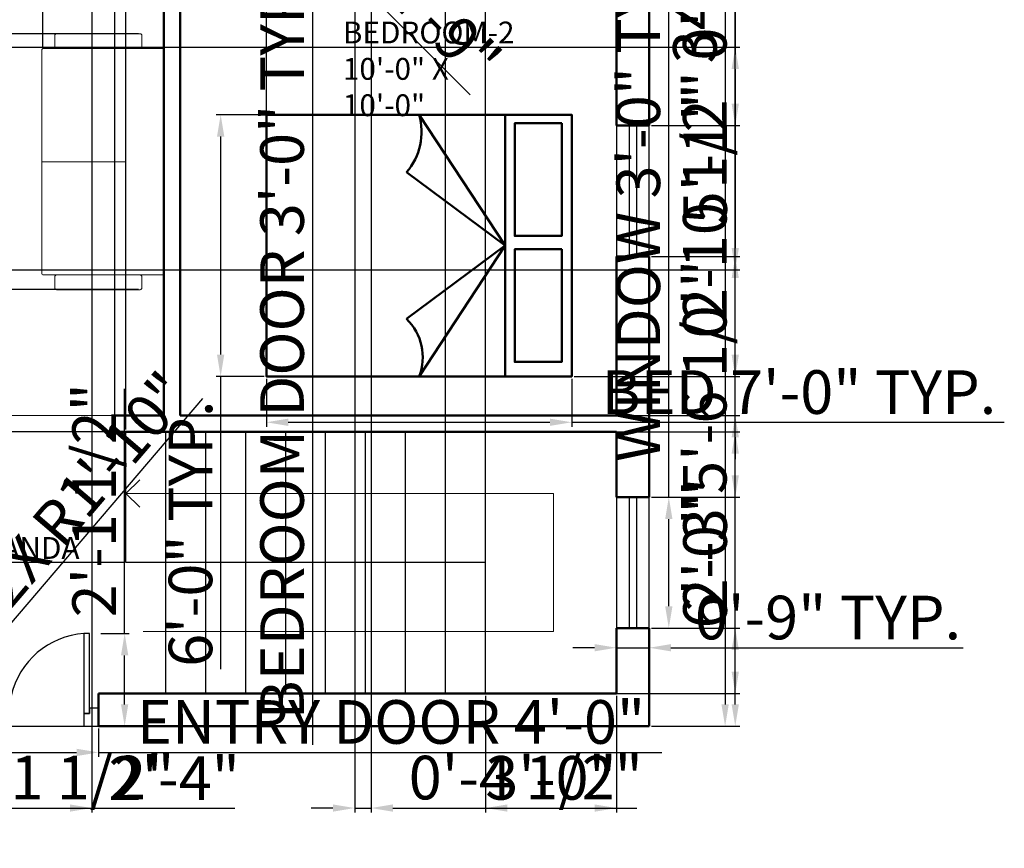
# Model space of a CAD drawing. Units: inches. Extents: x 1086 to 1501, y 383 to 973.
# Tile 2 of 7: x 1230 to 1501, y 383 to 611. Entities that reach past the tile are written whole.
import ezdxf

# ---------------------------------------------------------------- set-up
doc = ezdxf.new("R2010")
doc.units = ezdxf.units.IN
for name, color, linetype, lineweight in [('A-ANNO-DIMS', 2, 'Continuous', 18), ('A-ANNO-SYMB', 201, 'Continuous', 18), ('A-AREA-IDEN', 7, 'Continuous', 25), ('door', 10, 'Continuous', 25), ('furniture', 255, 'Continuous', 18), ('opening', 219, 'Continuous', 18), ('staircase', 201, 'Continuous', 25), ('wall', 7, 'Continuous', 50), ('window', 81, 'Continuous', 25)]:
    doc.layers.add(name, color=color, linetype=linetype, lineweight=lineweight)
doc.styles.get("Standard").update_dxf_attribs({"font": 'arial.ttf'})
doc.dimstyles.new('ISO-25', dxfattribs={"dimtxt": 12, "dimasz": 6, "dimexe": 1.25, "dimexo": 0.625, "dimtad": 1, "dimdec": 1, "dimlunit": 3, "dimtxsty": 'Standard', "dimcen": 2.5, "dimadec": 0, "dimazin": 0, "dimtfac": 1, "dimtdec": 1, "dimtmove": 0, "dimatfit": 3, "dimfxl": 1, "dimarcsym": 0})

# ---------------------------------------------------------------- blocks, each defined once
blk = doc.blocks.new('d3')
at = {"layer": 'door'}
blk.add_line((1743.18, 564.73), (1791.18, 564.73), dxfattribs=at)
for points in [[(1745.68, 568.23), (1747.18, 568.23), (1747.18, 590.23), (1745.68, 590.23)], [(1787.18, 568.23), (1788.68, 568.23), (1788.68, 590.23), (1787.18, 590.23)]]:
    blk.add_lwpolyline(points, close=True, dxfattribs=at)
for points in [[(1747.18, 564.73), (1743.18, 564.73), (1743.18, 569.73), (1745.68, 569.73), (1745.68, 568.23), (1747.18, 568.23), (1747.18, 564.73)], [(1787.18, 564.73), (1791.18, 564.73), (1791.18, 569.73), (1788.68, 569.73), (1788.68, 568.23), (1787.18, 568.23), (1787.18, 564.73)]]:
    blk.add_lwpolyline(points, dxfattribs=at)
for centre, start, end in [((1745.68, 568.23), 12.8362, 86.0995), ((1788.68, 568.23), 93.9005, 167.1638)]:
    blk.add_arc(centre, 22.05, start, end, dxfattribs=at)
blk = doc.blocks.new('w1')
at = {"layer": 'window'}
for p, q in [((1475.33, 845.32), (1475.33, 809.32)), ((1477.33, 845.32), (1477.33, 809.32))]:
    blk.add_line(p, q, dxfattribs=at)
blk.add_lwpolyline([(1471.83, 809.32), (1480.83, 809.32), (1480.83, 845.32), (1471.83, 845.32)], close=True, dxfattribs=at)
blk = doc.blocks.new('bed')
at = {"layer": 'wall'}
for p, q in [((1549.71, 859.44), (1621.71, 859.44)), ((1585.71, 859.44), (1549.71, 835.76)), ((1585.71, 859.44), (1565.54, 832.3)), ((1585.71, 859.44), (1621.71, 835.76)), ((1585.71, 859.44), (1605.88, 832.3))]:
    blk.add_line(p, q, dxfattribs=at)
for points in [[(1549.71, 793.76), (1621.71, 793.76), (1621.71, 877.76), (1549.71, 877.76)], [(1552.04, 875), (1583.04, 875), (1583.04, 862.08), (1552.04, 862.08)], [(1586.71, 875), (1617.71, 875), (1617.71, 862.08), (1586.71, 862.08)]]:
    blk.add_lwpolyline(points, close=True, dxfattribs=at)
for centre, radius, start, end in [((1554.45, 819.53), 16.91, 49.0428, 106.2967), ((1616.39, 822.13), 14.63, 68.7093, 135.9513)]:
    blk.add_arc(centre, radius, start, end, dxfattribs=at)
blk = doc.blocks.new('*D10')
at = {"layer": 'A-ANNO-DIMS', "color": 0, "lineweight": -2, "transparency": 16777216}
for p, q in [((1404.05, 835.21), (1425.57, 835.21)), ((1424.32, 829.21), (1424.32, 422.21)), ((1404.05, 416.21), (1425.57, 416.21))]:
    blk.add_line(p, q, dxfattribs=at)
at = {"layer": 'A-ANNO-DIMS', "color": 0, "transparency": 16777216}
for points in [[(1423.32, 829.21), (1425.32, 829.21), (1424.32, 835.21)], [(1423.32, 422.21), (1425.32, 422.21), (1424.32, 416.21)]]:
    blk.add_solid(points, dxfattribs=at)
at = {"layer": 'Defpoints', "color": 0, "transparency": 16777216}
for p in [(1403.43, 835.21), (1403.43, 416.21), (1424.32, 416.21)]:
    blk.add_point(p, dxfattribs=at)
at = {"layer": 'A-ANNO-DIMS', "color": 0, "transparency": 16777216, "insert": (1417.56, 625.71), "char_height": 12, "attachment_point": 5, "rotation": 90}
blk.add_mtext('34\'-11"', dxfattribs=at)
blk = doc.blocks.new('*D13')
at = {"layer": 'A-ANNO-DIMS', "color": 0, "lineweight": -2, "transparency": 16777216}
for p, q in [((1408.83, 479.21), (1408.83, 638.31)), ((1404.05, 479.21), (1410.08, 479.21)), ((1408.83, 449.21), (1408.83, 473.21)), ((1404.05, 443.21), (1410.08, 443.21))]:
    blk.add_line(p, q, dxfattribs=at)
at = {"layer": 'A-ANNO-DIMS', "color": 0, "transparency": 16777216}
for points in [[(1407.83, 473.21), (1409.83, 473.21), (1408.83, 479.21)], [(1407.83, 449.21), (1409.83, 449.21), (1408.83, 443.21)]]:
    blk.add_solid(points, dxfattribs=at)
at = {"layer": 'Defpoints', "color": 0, "transparency": 16777216}
for p in [(1403.43, 479.21), (1408.83, 479.21), (1403.43, 443.21)]:
    blk.add_point(p, dxfattribs=at)
at = {"layer": 'A-ANNO-DIMS', "color": 0, "transparency": 16777216, "insert": (1401.99, 561.76), "char_height": 12, "attachment_point": 5, "rotation": 90}
blk.add_mtext('WINDOW 3\'-0" TYP.', dxfattribs=at)
blk = doc.blocks.new('*D14')
at = {"layer": 'A-ANNO-DIMS', "color": 0, "lineweight": -2, "transparency": 16777216}
for p, q in [((1394.43, 442.58), (1394.43, 436.56)), ((1403.43, 442.58), (1403.43, 436.56)), ((1388.43, 437.81), (1382.43, 437.81)), ((1394.43, 437.81), (1403.43, 437.81)), ((1409.43, 437.81), (1489.83, 437.81))]:
    blk.add_line(p, q, dxfattribs=at)
at = {"layer": 'A-ANNO-DIMS', "color": 0, "transparency": 16777216}
for points in [[(1388.43, 438.81), (1388.43, 436.81), (1394.43, 437.81)], [(1409.43, 438.81), (1409.43, 436.81), (1403.43, 437.81)]]:
    blk.add_solid(points, dxfattribs=at)
at = {"layer": 'Defpoints', "color": 0, "transparency": 16777216}
for p in [(1394.43, 443.21), (1403.43, 443.21), (1403.43, 437.81)]:
    blk.add_point(p, dxfattribs=at)
at = {"layer": 'A-ANNO-DIMS', "color": 0, "transparency": 16777216, "insert": (1452.63, 444.56), "char_height": 12, "attachment_point": 5}
blk.add_mtext('0\'-9" TYP.', dxfattribs=at)
blk = doc.blocks.new('*D19')
at = {"layer": 'A-ANNO-DIMS', "color": 0, "lineweight": -2, "transparency": 16777216}
for p, q in [((1306.05, 673.21), (1312.08, 673.21)), ((1310.83, 667.21), (1310.83, 643.21)), ((1306.05, 637.21), (1312.08, 637.21)), ((1310.83, 637.21), (1310.83, 411.12))]:
    blk.add_line(p, q, dxfattribs=at)
at = {"layer": 'A-ANNO-DIMS', "color": 0, "transparency": 16777216}
for points in [[(1309.83, 667.21), (1311.83, 667.21), (1310.83, 673.21)], [(1309.83, 643.21), (1311.83, 643.21), (1310.83, 637.21)]]:
    blk.add_solid(points, dxfattribs=at)
at = {"layer": 'Defpoints', "color": 0, "transparency": 16777216}
for p in [(1305.43, 673.21), (1305.43, 637.21), (1310.83, 637.21)]:
    blk.add_point(p, dxfattribs=at)
at = {"layer": 'A-ANNO-DIMS', "color": 0, "transparency": 16777216, "insert": (1303.99, 521.16), "char_height": 12, "attachment_point": 5, "rotation": 90}
blk.add_mtext('BEDROOM DOOR 3\'-0" TYP.', dxfattribs=at)
blk = doc.blocks.new('*D21')
at = {"layer": 'A-ANNO-DIMS', "color": 0, "lineweight": -2, "transparency": 16777216}
for p, q in [((1203.93, 415.58), (1203.93, 407.76)), ((1251.93, 415.58), (1251.93, 407.76)), ((1209.93, 409.01), (1245.93, 409.01)), ((1251.93, 409.01), (1406.87, 409.01))]:
    blk.add_line(p, q, dxfattribs=at)
at = {"layer": 'A-ANNO-DIMS', "color": 0, "transparency": 16777216}
for points in [[(1209.93, 410.01), (1209.93, 408.01), (1203.93, 409.01)], [(1245.93, 410.01), (1245.93, 408.01), (1251.93, 409.01)]]:
    blk.add_solid(points, dxfattribs=at)
at = {"layer": 'Defpoints', "color": 0, "transparency": 16777216}
for p in [(1203.93, 416.21), (1251.93, 416.21), (1251.93, 409.01)]:
    blk.add_point(p, dxfattribs=at)
at = {"layer": 'A-ANNO-DIMS', "color": 0, "transparency": 16777216, "insert": (1332.4, 415.84), "char_height": 12, "attachment_point": 5}
blk.add_mtext('ENTRY DOOR 4\'-0"', dxfattribs=at)
blk = doc.blocks.new('*D22')
at = {"layer": 'A-ANNO-DIMS', "color": 0, "lineweight": -2, "transparency": 16777216}
for p, q in [((1259.13, 441.71), (1259.13, 509.02)), ((1252.55, 441.71), (1260.38, 441.71)), ((1259.13, 422.21), (1259.13, 435.71)), ((1252.55, 416.21), (1260.38, 416.21))]:
    blk.add_line(p, q, dxfattribs=at)
at = {"layer": 'A-ANNO-DIMS', "color": 0, "transparency": 16777216}
for points in [[(1258.13, 435.71), (1260.13, 435.71), (1259.13, 441.71)], [(1258.13, 422.21), (1260.13, 422.21), (1259.13, 416.21)]]:
    blk.add_solid(points, dxfattribs=at)
at = {"layer": 'Defpoints', "color": 0, "transparency": 16777216}
for p in [(1251.93, 441.71), (1259.13, 441.71), (1251.93, 416.21)]:
    blk.add_point(p, dxfattribs=at)
at = {"layer": 'A-ANNO-DIMS', "color": 0, "transparency": 16777216, "insert": (1252.3, 478.36), "char_height": 12, "attachment_point": 5, "rotation": 90}
blk.add_mtext('2\'-1 1/2"', dxfattribs=at)
blk = doc.blocks.new('*D23')
at = {"layer": 'A-ANNO-DIMS', "color": 0, "lineweight": -2, "transparency": 16777216}
for p, q in [((1298.14, 511.79), (1298.14, 498.57)), ((1382.14, 511.79), (1382.14, 498.57)), ((1304.14, 499.82), (1376.14, 499.82)), ((1382.14, 499.82), (1501.13, 499.82))]:
    blk.add_line(p, q, dxfattribs=at)
at = {"layer": 'A-ANNO-DIMS', "color": 0, "transparency": 16777216}
for points in [[(1304.14, 500.82), (1304.14, 498.82), (1298.14, 499.82)], [(1376.14, 500.82), (1376.14, 498.82), (1382.14, 499.82)]]:
    blk.add_solid(points, dxfattribs=at)
at = {"layer": 'Defpoints', "color": 0, "transparency": 16777216}
for p in [(1298.14, 512.42), (1382.14, 512.42), (1382.14, 499.82)]:
    blk.add_point(p, dxfattribs=at)
at = {"layer": 'A-ANNO-DIMS', "color": 0, "transparency": 16777216, "insert": (1444.63, 506.57), "char_height": 12, "attachment_point": 5}
blk.add_mtext('BED 7\'-0" TYP.', dxfattribs=at)
blk = doc.blocks.new('*D24')
at = {"layer": 'A-ANNO-DIMS', "color": 0, "lineweight": -2, "transparency": 16777216}
for p, q in [((1297.51, 584.42), (1284.29, 584.42)), ((1285.54, 578.42), (1285.54, 518.42)), ((1297.51, 512.42), (1284.29, 512.42)), ((1285.54, 512.42), (1285.54, 431.95))]:
    blk.add_line(p, q, dxfattribs=at)
at = {"layer": 'A-ANNO-DIMS', "color": 0, "transparency": 16777216}
for points in [[(1284.54, 578.42), (1286.54, 578.42), (1285.54, 584.42)], [(1284.54, 518.42), (1286.54, 518.42), (1285.54, 512.42)]]:
    blk.add_solid(points, dxfattribs=at)
at = {"layer": 'Defpoints', "color": 0, "transparency": 16777216}
for p in [(1298.14, 584.42), (1285.54, 512.42), (1298.14, 512.42)]:
    blk.add_point(p, dxfattribs=at)
at = {"layer": 'A-ANNO-DIMS', "color": 0, "transparency": 16777216, "insert": (1278.79, 469.18), "char_height": 12, "attachment_point": 5, "rotation": 90}
blk.add_mtext('6\'-0" TYP.', dxfattribs=at)
blk = doc.blocks.new('*D34')
at = {"layer": 'A-ANNO-DIMS', "color": 0, "lineweight": -2, "transparency": 16777216}
for p, q in [((1427.11, 443.21), (1427.11, 482.56)), ((1404.05, 443.21), (1428.36, 443.21)), ((1427.11, 422.21), (1427.11, 437.21)), ((1404.05, 416.21), (1428.36, 416.21))]:
    blk.add_line(p, q, dxfattribs=at)
at = {"layer": 'A-ANNO-DIMS', "color": 0, "transparency": 16777216}
for points in [[(1426.11, 437.21), (1428.11, 437.21), (1427.11, 443.21)], [(1426.11, 422.21), (1428.11, 422.21), (1427.11, 416.21)]]:
    blk.add_solid(points, dxfattribs=at)
at = {"layer": 'Defpoints', "color": 0, "transparency": 16777216}
for p in [(1403.43, 443.21), (1427.11, 443.21), (1403.43, 416.21)]:
    blk.add_point(p, dxfattribs=at)
at = {"layer": 'A-ANNO-DIMS', "color": 0, "transparency": 16777216, "insert": (1420.36, 465.88), "char_height": 12, "attachment_point": 5, "rotation": 90}
blk.add_mtext('2\'-3"', dxfattribs=at)
blk = doc.blocks.new('*D35')
at = {"layer": 'A-ANNO-DIMS', "color": 0, "lineweight": -2, "transparency": 16777216}
for p, q in [((1404.05, 545.46), (1428.36, 545.46)), ((1427.11, 485.21), (1427.11, 539.46)), ((1404.05, 479.21), (1428.36, 479.21))]:
    blk.add_line(p, q, dxfattribs=at)
at = {"layer": 'A-ANNO-DIMS', "color": 0, "transparency": 16777216}
for points in [[(1426.11, 539.46), (1428.11, 539.46), (1427.11, 545.46)], [(1426.11, 485.21), (1428.11, 485.21), (1427.11, 479.21)]]:
    blk.add_solid(points, dxfattribs=at)
at = {"layer": 'Defpoints', "color": 0, "transparency": 16777216}
for p in [(1403.43, 545.46), (1427.11, 545.46), (1403.43, 479.21)]:
    blk.add_point(p, dxfattribs=at)
at = {"layer": 'A-ANNO-DIMS', "color": 0, "transparency": 16777216, "insert": (1420.28, 512.33), "char_height": 12, "attachment_point": 5, "rotation": 90}
blk.add_mtext('5\'-6 1/2"', dxfattribs=at)
blk = doc.blocks.new('*D36')
at = {"layer": 'A-ANNO-DIMS', "color": 0, "lineweight": -2, "transparency": 16777216}
for p, q in [((1427.11, 641.71), (1427.11, 708.82)), ((1404.05, 641.71), (1428.36, 641.71)), ((1427.11, 587.46), (1427.11, 635.71)), ((1404.05, 581.46), (1428.36, 581.46))]:
    blk.add_line(p, q, dxfattribs=at)
at = {"layer": 'A-ANNO-DIMS', "color": 0, "transparency": 16777216}
for points in [[(1426.11, 635.71), (1428.11, 635.71), (1427.11, 641.71)], [(1426.11, 587.46), (1428.11, 587.46), (1427.11, 581.46)]]:
    blk.add_solid(points, dxfattribs=at)
at = {"layer": 'Defpoints', "color": 0, "transparency": 16777216}
for p in [(1403.43, 641.71), (1427.11, 641.71), (1403.43, 581.46)]:
    blk.add_point(p, dxfattribs=at)
at = {"layer": 'A-ANNO-DIMS', "color": 0, "transparency": 16777216, "insert": (1420.28, 678.26), "char_height": 12, "attachment_point": 5, "rotation": 90}
blk.add_mtext('5\'-0 1/2"', dxfattribs=at)
blk = doc.blocks.new('*D39')
at = {"layer": 'A-ANNO-DIMS', "color": 0, "lineweight": -2, "transparency": 16777216}
for p, q in [((1178.43, 415.58), (1178.43, 392.46)), ((1203.93, 415.58), (1203.93, 392.46)), ((1184.43, 393.71), (1197.93, 393.71)), ((1203.93, 393.71), (1271.25, 393.71))]:
    blk.add_line(p, q, dxfattribs=at)
at = {"layer": 'A-ANNO-DIMS', "color": 0, "transparency": 16777216}
for points in [[(1184.43, 394.71), (1184.43, 392.71), (1178.43, 393.71)], [(1197.93, 394.71), (1197.93, 392.71), (1203.93, 393.71)]]:
    blk.add_solid(points, dxfattribs=at)
at = {"layer": 'Defpoints', "color": 0, "transparency": 16777216}
for p in [(1178.43, 416.21), (1203.93, 416.21), (1203.93, 393.71)]:
    blk.add_point(p, dxfattribs=at)
at = {"layer": 'A-ANNO-DIMS', "color": 0, "transparency": 16777216, "insert": (1240.59, 400.54), "char_height": 12, "attachment_point": 5}
blk.add_mtext('2\'-1 1/2"', dxfattribs=at)
blk = doc.blocks.new('*D40')
at = {"layer": 'A-ANNO-DIMS', "color": 0, "lineweight": -2, "transparency": 16777216}
for p, q in [((1142.43, 502.33), (1142.43, 867.19)), ((1269.93, 502.33), (1269.93, 867.19)), ((1148.43, 865.94), (1263.93, 865.94))]:
    blk.add_line(p, q, dxfattribs=at)
at = {"layer": 'A-ANNO-DIMS', "color": 0, "transparency": 16777216}
for points in [[(1148.43, 866.94), (1148.43, 864.94), (1142.43, 865.94)], [(1263.93, 866.94), (1263.93, 864.94), (1269.93, 865.94)]]:
    blk.add_solid(points, dxfattribs=at)
at = {"layer": 'Defpoints', "color": 0, "transparency": 16777216}
for p in [(1269.93, 865.94), (1142.43, 501.71), (1269.93, 501.71)]:
    blk.add_point(p, dxfattribs=at)
at = {"layer": 'A-ANNO-DIMS', "color": 0, "transparency": 16777216, "insert": (1206.18, 872.77), "char_height": 12, "attachment_point": 5}
blk.add_mtext('10\'-7 1/2"', dxfattribs=at)
blk = doc.blocks.new('*D42')
at = {"layer": 'A-ANNO-DIMS', "color": 0, "lineweight": -2, "transparency": 16777216}
for p, q in [((1256.43, 502.33), (1256.43, 867.19)), ((1269.93, 502.33), (1269.93, 867.19)), ((1262.43, 865.94), (1263.93, 865.94)), ((1269.93, 865.94), (1335.91, 865.94))]:
    blk.add_line(p, q, dxfattribs=at)
at = {"layer": 'A-ANNO-DIMS', "color": 0, "transparency": 16777216}
for points in [[(1262.43, 866.94), (1262.43, 864.94), (1256.43, 865.94)], [(1263.93, 866.94), (1263.93, 864.94), (1269.93, 865.94)]]:
    blk.add_solid(points, dxfattribs=at)
at = {"layer": 'Defpoints', "color": 0, "transparency": 16777216}
for p in [(1269.93, 865.94), (1256.43, 501.71), (1269.93, 501.71)]:
    blk.add_point(p, dxfattribs=at)
at = {"layer": 'A-ANNO-DIMS', "color": 0, "transparency": 16777216, "insert": (1305.92, 872.77), "char_height": 12, "attachment_point": 5}
blk.add_mtext('1\'-1 1/2"', dxfattribs=at)
blk = doc.blocks.new('*D43')
at = {"layer": 'A-ANNO-DIMS', "color": 0, "lineweight": -2, "transparency": 16777216}
for p, q in [((1208.43, 497.83), (1208.43, 867.19)), ((1256.43, 497.83), (1256.43, 867.19)), ((1214.43, 865.94), (1250.43, 865.94))]:
    blk.add_line(p, q, dxfattribs=at)
at = {"layer": 'A-ANNO-DIMS', "color": 0, "transparency": 16777216}
for points in [[(1214.43, 866.94), (1214.43, 864.94), (1208.43, 865.94)], [(1250.43, 866.94), (1250.43, 864.94), (1256.43, 865.94)]]:
    blk.add_solid(points, dxfattribs=at)
at = {"layer": 'Defpoints', "color": 0, "transparency": 16777216}
for p in [(1256.43, 865.94), (1208.43, 497.21), (1256.43, 497.21)]:
    blk.add_point(p, dxfattribs=at)
at = {"layer": 'A-ANNO-DIMS', "color": 0, "transparency": 16777216, "insert": (1232.43, 872.69), "char_height": 12, "attachment_point": 5}
blk.add_mtext('4\'-0"', dxfattribs=at)
blk = doc.blocks.new('*D44')
at = {"layer": 'A-ANNO-DIMS', "color": 0, "lineweight": -2, "transparency": 16777216}
for p, q in [((1258.8, 497.21), (1109.68, 497.21)), ((1110.93, 491.21), (1110.93, 467.21)), ((1258.8, 461.21), (1109.68, 461.21))]:
    blk.add_line(p, q, dxfattribs=at)
at = {"layer": 'A-ANNO-DIMS', "color": 0, "transparency": 16777216}
for points in [[(1109.93, 491.21), (1111.93, 491.21), (1110.93, 497.21)], [(1109.93, 467.21), (1111.93, 467.21), (1110.93, 461.21)]]:
    blk.add_solid(points, dxfattribs=at)
at = {"layer": 'Defpoints', "color": 0, "transparency": 16777216}
for p in [(1259.43, 497.21), (1110.93, 461.21), (1259.43, 461.21)]:
    blk.add_point(p, dxfattribs=at)
at = {"layer": 'A-ANNO-DIMS', "color": 0, "transparency": 16777216, "insert": (1104.17, 479.21), "char_height": 12, "attachment_point": 5, "rotation": 90}
blk.add_mtext('3\'-0"', dxfattribs=at)
blk = doc.blocks.new('*D45')
at = {"layer": 'A-ANNO-DIMS', "color": 0, "lineweight": -2, "transparency": 16777216}
for p, q in [((1259.43, 497.83), (1259.43, 867.19)), ((1358.43, 497.83), (1358.43, 867.19)), ((1265.43, 865.94), (1352.43, 865.94))]:
    blk.add_line(p, q, dxfattribs=at)
at = {"layer": 'A-ANNO-DIMS', "color": 0, "transparency": 16777216}
for points in [[(1265.43, 866.94), (1265.43, 864.94), (1259.43, 865.94)], [(1352.43, 866.94), (1352.43, 864.94), (1358.43, 865.94)]]:
    blk.add_solid(points, dxfattribs=at)
at = {"layer": 'Defpoints', "color": 0, "transparency": 16777216}
for p in [(1358.43, 865.94), (1259.43, 497.21), (1358.43, 497.21)]:
    blk.add_point(p, dxfattribs=at)
at = {"layer": 'A-ANNO-DIMS', "color": 0, "transparency": 16777216, "insert": (1308.93, 872.7), "char_height": 12, "attachment_point": 5}
blk.add_mtext('8\'-3"', dxfattribs=at)
blk = doc.blocks.new('*D46')
at = {"layer": 'A-ANNO-DIMS', "color": 0, "lineweight": -2, "transparency": 16777216}
for p, q in [((1358.43, 424.58), (1358.43, 392.46)), ((1394.43, 424.58), (1394.43, 392.46)), ((1364.43, 393.71), (1388.43, 393.71))]:
    blk.add_line(p, q, dxfattribs=at)
at = {"layer": 'A-ANNO-DIMS', "color": 0, "transparency": 16777216}
for points in [[(1364.43, 394.71), (1364.43, 392.71), (1358.43, 393.71)], [(1388.43, 394.71), (1388.43, 392.71), (1394.43, 393.71)]]:
    blk.add_solid(points, dxfattribs=at)
at = {"layer": 'Defpoints', "color": 0, "transparency": 16777216}
for p in [(1358.43, 425.21), (1394.43, 425.21), (1394.43, 393.71)]:
    blk.add_point(p, dxfattribs=at)
at = {"layer": 'A-ANNO-DIMS', "color": 0, "transparency": 16777216, "insert": (1376.43, 400.46), "char_height": 12, "attachment_point": 5}
blk.add_mtext('3\'-0"', dxfattribs=at)
blk = doc.blocks.new('*D47')
at = {"layer": 'A-ANNO-DIMS', "color": 0, "lineweight": -2, "transparency": 16777216}
for p, q in [((1347.43, 425.83), (1347.43, 867.19)), ((1358.43, 425.83), (1358.43, 867.19)), ((1341.43, 865.94), (1335.43, 865.94)), ((1347.43, 865.94), (1358.43, 865.94)), ((1364.43, 865.94), (1412.9, 865.94))]:
    blk.add_line(p, q, dxfattribs=at)
at = {"layer": 'A-ANNO-DIMS', "color": 0, "transparency": 16777216}
for points in [[(1341.43, 866.94), (1341.43, 864.94), (1347.43, 865.94)], [(1364.43, 866.94), (1364.43, 864.94), (1358.43, 865.94)]]:
    blk.add_solid(points, dxfattribs=at)
at = {"layer": 'Defpoints', "color": 0, "transparency": 16777216}
for p in [(1358.43, 865.94), (1347.43, 425.21), (1358.43, 425.21)]:
    blk.add_point(p, dxfattribs=at)
at = {"layer": 'A-ANNO-DIMS', "color": 0, "transparency": 16777216, "insert": (1391.67, 872.69), "char_height": 12, "attachment_point": 5}
blk.add_mtext('0\'-11"', dxfattribs=at)
blk = doc.blocks.new('*D48')
at = {"layer": 'A-ANNO-DIMS', "color": 0, "lineweight": -2, "transparency": 16777216}
for p, q in [((1359.05, 497.21), (1428.36, 497.21)), ((1427.11, 431.21), (1427.11, 491.21)), ((1359.05, 425.21), (1428.36, 425.21))]:
    blk.add_line(p, q, dxfattribs=at)
at = {"layer": 'A-ANNO-DIMS', "color": 0, "transparency": 16777216}
for points in [[(1426.11, 491.21), (1428.11, 491.21), (1427.11, 497.21)], [(1426.11, 431.21), (1428.11, 431.21), (1427.11, 425.21)]]:
    blk.add_solid(points, dxfattribs=at)
at = {"layer": 'Defpoints', "color": 0, "transparency": 16777216}
for p in [(1358.43, 497.21), (1427.11, 497.21), (1358.43, 425.21)]:
    blk.add_point(p, dxfattribs=at)
at = {"layer": 'A-ANNO-DIMS', "color": 0, "transparency": 16777216, "insert": (1420.36, 461.21), "char_height": 12, "attachment_point": 5, "rotation": 90}
blk.add_mtext('6\'-0"', dxfattribs=at)
blk = doc.blocks.new('*D50')
at = {"layer": 'A-ANNO-DIMS', "color": 0, "lineweight": -2, "transparency": 16777216}
for p, q in [((1184.43, 502.33), (1184.43, 867.19)), ((1208.43, 502.33), (1208.43, 867.19)), ((1190.43, 865.94), (1202.43, 865.94)), ((1208.43, 865.94), (1247.78, 865.94))]:
    blk.add_line(p, q, dxfattribs=at)
at = {"layer": 'A-ANNO-DIMS', "color": 0, "transparency": 16777216}
for points in [[(1190.43, 866.94), (1190.43, 864.94), (1184.43, 865.94)], [(1202.43, 866.94), (1202.43, 864.94), (1208.43, 865.94)]]:
    blk.add_solid(points, dxfattribs=at)
at = {"layer": 'Defpoints', "color": 0, "transparency": 16777216}
for p in [(1208.43, 865.94), (1184.43, 501.71), (1208.43, 501.71)]:
    blk.add_point(p, dxfattribs=at)
at = {"layer": 'A-ANNO-DIMS', "color": 0, "transparency": 16777216, "insert": (1231.11, 872.69), "char_height": 12, "attachment_point": 5}
blk.add_mtext('2\'-0"', dxfattribs=at)
blk = doc.blocks.new('*D58')
at = {"layer": 'A-ANNO-DIMS', "color": 0, "lineweight": -2, "transparency": 16777216}
for p, q in [((1250.08, 809.82), (1250.08, 392.46)), ((1222.08, 799.32), (1222.08, 392.46)), ((1228.08, 393.71), (1244.08, 393.71)), ((1250.08, 393.71), (1289.44, 393.71))]:
    blk.add_line(p, q, dxfattribs=at)
at = {"layer": 'A-ANNO-DIMS', "color": 0, "transparency": 16777216}
for points in [[(1228.08, 394.71), (1228.08, 392.71), (1222.08, 393.71)], [(1244.08, 394.71), (1244.08, 392.71), (1250.08, 393.71)]]:
    blk.add_solid(points, dxfattribs=at)
at = {"layer": 'Defpoints', "color": 0, "transparency": 16777216}
for p in [(1250.08, 810.44), (1222.08, 799.94), (1250.08, 393.71)]:
    blk.add_point(p, dxfattribs=at)
at = {"layer": 'A-ANNO-DIMS', "color": 0, "transparency": 16777216, "insert": (1272.76, 400.36), "char_height": 12, "attachment_point": 5}
blk.add_mtext('2\'-4"', dxfattribs=at)
blk = doc.blocks.new('*D60')
at = {"layer": 'A-ANNO-DIMS', "color": 0, "lineweight": -2, "transparency": 16777216}
for p, q in [((1322.43, 629.08), (1322.43, 392.46)), ((1326.93, 629.08), (1326.93, 392.46)), ((1316.43, 393.71), (1310.43, 393.71)), ((1322.43, 393.71), (1326.93, 393.71)), ((1332.93, 393.71), (1400.04, 393.71))]:
    blk.add_line(p, q, dxfattribs=at)
at = {"layer": 'A-ANNO-DIMS', "color": 0, "transparency": 16777216}
for points in [[(1316.43, 394.71), (1316.43, 392.71), (1322.43, 393.71)], [(1332.93, 394.71), (1332.93, 392.71), (1326.93, 393.71)]]:
    blk.add_solid(points, dxfattribs=at)
at = {"layer": 'Defpoints', "color": 0, "transparency": 16777216}
for p in [(1322.43, 629.71), (1326.93, 629.71), (1326.93, 393.71)]:
    blk.add_point(p, dxfattribs=at)
at = {"layer": 'A-ANNO-DIMS', "color": 0, "transparency": 16777216, "insert": (1369.49, 400.54), "char_height": 12, "attachment_point": 5}
blk.add_mtext('0\'-4 1/2"', dxfattribs=at)
blk = doc.blocks.new('*D62')
at = {"layer": 'A-ANNO-DIMS', "color": 0, "lineweight": -2, "transparency": 16777216}
for p, q in [((1427.11, 683.71), (1427.11, 689.71)), ((1395.05, 677.71), (1428.36, 677.71)), ((1427.11, 677.71), (1427.11, 674.06)), ((1382.74, 674.06), (1428.36, 674.06)), ((1427.11, 668.06), (1427.11, 600.95))]:
    blk.add_line(p, q, dxfattribs=at)
at = {"layer": 'A-ANNO-DIMS', "color": 0, "transparency": 16777216}
for points in [[(1426.11, 683.71), (1428.11, 683.71), (1427.11, 677.71)], [(1426.11, 668.06), (1428.11, 668.06), (1427.11, 674.06)]]:
    blk.add_solid(points, dxfattribs=at)
at = {"layer": 'Defpoints', "color": 0, "transparency": 16777216}
for p in [(1394.43, 677.71), (1382.11, 674.06), (1427.11, 674.06)]:
    blk.add_point(p, dxfattribs=at)
at = {"layer": 'A-ANNO-DIMS', "color": 0, "transparency": 16777216, "insert": (1420.28, 631.51), "char_height": 12, "attachment_point": 5, "rotation": 90}
blk.add_mtext('0\'-3 1/2"', dxfattribs=at)
blk = doc.blocks.new('*D68')
at = {"layer": 'A-ANNO-DIMS', "color": 0, "lineweight": -2, "transparency": 16777216}
for p, q in [((1110.93, 606.65), (1110.93, 683.08)), ((1262.93, 606.65), (1109.68, 606.65)), ((1110.93, 542.31), (1110.93, 600.65)), ((1262.93, 536.31), (1109.68, 536.31))]:
    blk.add_line(p, q, dxfattribs=at)
at = {"layer": 'A-ANNO-DIMS', "color": 0, "transparency": 16777216}
for points in [[(1109.93, 600.65), (1111.93, 600.65), (1110.93, 606.65)], [(1109.93, 542.31), (1111.93, 542.31), (1110.93, 536.31)]]:
    blk.add_solid(points, dxfattribs=at)
at = {"layer": 'Defpoints', "color": 0, "transparency": 16777216}
for p in [(1110.93, 606.65), (1263.55, 606.65), (1263.55, 536.31)]:
    blk.add_point(p, dxfattribs=at)
at = {"layer": 'A-ANNO-DIMS', "color": 0, "transparency": 16777216, "insert": (1104.1, 647.86), "char_height": 12, "attachment_point": 5, "rotation": 90}
blk.add_mtext('5\'-10 1/2"', dxfattribs=at)
blk = doc.blocks.new('*D69')
at = {"layer": 'A-ANNO-DIMS', "color": 0, "lineweight": -2, "transparency": 16777216}
for p, q in [((1236.63, 603.21), (1236.63, 867.19)), ((1269.93, 603.25), (1269.93, 867.19)), ((1242.63, 865.94), (1263.93, 865.94)), ((1269.93, 865.94), (1337.25, 865.94))]:
    blk.add_line(p, q, dxfattribs=at)
at = {"layer": 'A-ANNO-DIMS', "color": 0, "transparency": 16777216}
for points in [[(1242.63, 866.94), (1242.63, 864.94), (1236.63, 865.94)], [(1263.93, 866.94), (1263.93, 864.94), (1269.93, 865.94)]]:
    blk.add_solid(points, dxfattribs=at)
at = {"layer": 'Defpoints', "color": 0, "transparency": 16777216}
for p in [(1269.93, 865.94), (1236.63, 602.59), (1269.93, 602.62)]:
    blk.add_point(p, dxfattribs=at)
at = {"layer": 'A-ANNO-DIMS', "color": 0, "transparency": 16777216, "insert": (1306.59, 872.77), "char_height": 12, "attachment_point": 5}
blk.add_mtext('2\'-9 1/2"', dxfattribs=at)
blk = doc.blocks.new('*D70')
at = {"layer": 'A-ANNO-DIMS', "color": 0, "lineweight": -2, "transparency": 16777216}
for p, q in [((1269.3, 637.21), (1109.68, 637.21)), ((1110.93, 631.21), (1110.93, 612.65)), ((1262.93, 606.65), (1109.68, 606.65)), ((1110.93, 606.65), (1110.93, 539.33))]:
    blk.add_line(p, q, dxfattribs=at)
at = {"layer": 'A-ANNO-DIMS', "color": 0, "transparency": 16777216}
for points in [[(1109.93, 631.21), (1111.93, 631.21), (1110.93, 637.21)], [(1109.93, 612.65), (1111.93, 612.65), (1110.93, 606.65)]]:
    blk.add_solid(points, dxfattribs=at)
at = {"layer": 'Defpoints', "color": 0, "transparency": 16777216}
for p in [(1269.93, 637.21), (1110.93, 606.65), (1263.55, 606.65)]:
    blk.add_point(p, dxfattribs=at)
at = {"layer": 'A-ANNO-DIMS', "color": 0, "transparency": 16777216, "insert": (1104.1, 569.99), "char_height": 12, "attachment_point": 5, "rotation": 90}
blk.add_mtext('2\'-6 1/2"', dxfattribs=at)
blk = doc.blocks.new('*D72')
at = {"layer": 'A-ANNO-DIMS', "color": 0, "lineweight": -2, "transparency": 16777216}
for p, q in [((1149.81, 602.97), (1428.36, 602.97)), ((1427.11, 596.97), (1427.11, 547.72)), ((1149.81, 541.72), (1428.36, 541.72))]:
    blk.add_line(p, q, dxfattribs=at)
at = {"layer": 'A-ANNO-DIMS', "color": 0, "transparency": 16777216}
for points in [[(1426.11, 596.97), (1428.11, 596.97), (1427.11, 602.97)], [(1426.11, 547.72), (1428.11, 547.72), (1427.11, 541.72)]]:
    blk.add_solid(points, dxfattribs=at)
at = {"layer": 'Defpoints', "color": 0, "transparency": 16777216}
for p in [(1149.18, 602.97), (1149.18, 541.72), (1427.11, 541.72)]:
    blk.add_point(p, dxfattribs=at)
at = {"layer": 'A-ANNO-DIMS', "color": 0, "transparency": 16777216, "insert": (1420.36, 572.35), "char_height": 12, "attachment_point": 5, "rotation": 90}
blk.add_mtext('5\'-1"', dxfattribs=at)
blk = doc.blocks.new('*D76')
at = {"layer": 'A-ANNO-DIMS', "color": 0, "lineweight": -2, "transparency": 16777216}
for p, q in [((1427.11, 518.42), (1427.11, 594.85)), ((1382.76, 512.42), (1428.36, 512.42)), ((1427.11, 501.71), (1427.11, 512.42)), ((1395.05, 501.71), (1428.36, 501.71)), ((1427.11, 495.71), (1427.11, 489.71))]:
    blk.add_line(p, q, dxfattribs=at)
at = {"layer": 'A-ANNO-DIMS', "color": 0, "transparency": 16777216}
for points in [[(1426.11, 518.42), (1428.11, 518.42), (1427.11, 512.42)], [(1426.11, 495.71), (1428.11, 495.71), (1427.11, 501.71)]]:
    blk.add_solid(points, dxfattribs=at)
at = {"layer": 'Defpoints', "color": 0, "transparency": 16777216}
for p in [(1382.14, 512.42), (1427.11, 512.42), (1394.43, 501.71)]:
    blk.add_point(p, dxfattribs=at)
at = {"layer": 'A-ANNO-DIMS', "color": 0, "transparency": 16777216, "insert": (1420.28, 559.63), "char_height": 12, "attachment_point": 5, "rotation": 90}
blk.add_mtext('0\'-10 1/2"', dxfattribs=at)
blk = doc.blocks.new('*D77')
at = {"layer": 'A-ANNO-DIMS', "color": 0, "lineweight": -2, "transparency": 16777216}
for p, q in [((1274.43, 502.33), (1274.43, 867.19)), ((1298.14, 513.04), (1298.14, 867.19)), ((1280.43, 865.94), (1292.14, 865.94)), ((1298.14, 865.94), (1373.44, 865.94))]:
    blk.add_line(p, q, dxfattribs=at)
at = {"layer": 'A-ANNO-DIMS', "color": 0, "transparency": 16777216}
for points in [[(1280.43, 866.94), (1280.43, 864.94), (1274.43, 865.94)], [(1292.14, 866.94), (1292.14, 864.94), (1298.14, 865.94)]]:
    blk.add_solid(points, dxfattribs=at)
at = {"layer": 'Defpoints', "color": 0, "transparency": 16777216}
for p in [(1298.14, 865.94), (1298.14, 512.42), (1274.43, 501.71)]:
    blk.add_point(p, dxfattribs=at)
at = {"layer": 'A-ANNO-DIMS', "color": 0, "transparency": 16777216, "insert": (1338.79, 872.77), "char_height": 12, "attachment_point": 5}
blk.add_mtext('1\'-11 1/2"', dxfattribs=at)
blk = doc.blocks.new('*D78')
at = {"layer": 'A-ANNO-DIMS', "color": 0, "lineweight": -2, "transparency": 16777216}
for p, q in [((1272.43, 671.71), (1295.79, 648.35)), ((1354.21, 589.92), (1300.03, 644.11))]:
    blk.add_line(p, q, dxfattribs=at)
at = {"layer": 'A-ANNO-DIMS', "color": 0, "transparency": 16777216}
blk.add_solid([(1300.74, 644.81), (1299.32, 643.4), (1295.79, 648.35)], dxfattribs=at)
at = {"layer": 'Defpoints', "color": 0, "transparency": 16777216}
for p in [(1272.43, 671.71), (1295.79, 648.35)]:
    blk.add_point(p, dxfattribs=at)
at = {"layer": 'A-ANNO-DIMS', "color": 0, "transparency": 16777216, "insert": (1334.02, 619.67), "char_height": 12, "attachment_point": 5, "rotation": 314.9994}
blk.add_mtext('2X R2\'-9"', dxfattribs=at)
blk = doc.blocks.new('*D80')
at = {"layer": 'A-ANNO-DIMS', "color": 0, "lineweight": -2, "transparency": 16777216}
for p, q in [((1280.51, 506.35), (1224.66, 441.03)), ((1206.43, 419.71), (1220.76, 436.47))]:
    blk.add_line(p, q, dxfattribs=at)
at = {"layer": 'A-ANNO-DIMS', "color": 0, "transparency": 16777216}
blk.add_solid([(1223.9, 441.68), (1225.42, 440.38), (1220.76, 436.47)], dxfattribs=at)
at = {"layer": 'Defpoints', "color": 0, "transparency": 16777216}
for p in [(1220.76, 436.47), (1206.43, 419.71)]:
    blk.add_point(p, dxfattribs=at)
at = {"layer": 'A-ANNO-DIMS', "color": 0, "transparency": 16777216, "insert": (1249.4, 480.36), "char_height": 12, "attachment_point": 5, "rotation": 49.4689}
blk.add_mtext('2X R1\'-10"', dxfattribs=at)

msp = doc.modelspace()

# ---------------------------------------------------------------- linework, layer by layer
at = {"layer": 'A-ANNO-SYMB'}
for p, q in [((1259.43, 480.2), (1263.33, 483.95)), ((1377.09, 480.2), (1259.43, 480.2)), ((1259.43, 480.2), (1263.33, 476.46)), ((1377.09, 442.23), (1377.09, 480.2)), ((1264.19, 442.23), (1377.09, 442.23))]:
    msp.add_line(p, q, dxfattribs=at)
at = {"layer": 'furniture'}
msp.add_line((1259.32, 571.48), (1236.32, 571.48), dxfattribs=at)
for points in [[(1263.86, 603.12), (1263.86, 606.18, 0.414214), (1263.36, 606.68), (1240.42, 606.68, 0.414214), (1239.92, 606.18), (1239.92, 603.12, 0.414214), (1240.42, 602.62), (1263.36, 602.62, 0.414214)], [(1263.86, 536.78), (1263.86, 539.83, 0.414214), (1263.36, 540.33), (1236.82, 540.33, -0.414214), (1236.32, 540.83), (1236.32, 602.12, -0.414214), (1236.82, 602.62), (1259.32, 602.62), (1259.32, 540.33), (1240.42, 540.33, 0.414214), (1239.92, 539.83), (1239.92, 536.78, 0.414214), (1240.42, 536.28), (1263.36, 536.28, 0.414214)]]:
    msp.add_lwpolyline(points, format="xyb", close=True, dxfattribs=at)
msp.add_lwpolyline([(1269.93, 602.62), (1259.32, 602.62), (1259.32, 540.33), (1269.93, 540.33)], close=True, dxfattribs=at)
at = {"layer": 'opening'}
msp.add_lwpolyline([(1208.43, 501.71), (1256.43, 501.71), (1256.43, 497.21), (1208.43, 497.21)], close=True, dxfattribs=at)
at = {"layer": 'staircase'}
for p, q in [((1259.43, 461.21), (1259.43, 497.21)), ((1270.43, 425.21), (1270.43, 497.21)), ((1281.43, 425.21), (1281.43, 497.21)), ((1292.43, 425.21), (1292.43, 497.21)), ((1303.43, 425.21), (1303.43, 497.21)), ((1314.43, 425.21), (1314.43, 497.21)), ((1325.43, 425.21), (1325.43, 497.21)), ((1336.43, 425.21), (1336.43, 497.21)), ((1347.43, 425.21), (1347.43, 497.21)), ((1358.43, 425.21), (1358.43, 497.21)), ((1358.43, 461.21), (1259.43, 461.21))]:
    msp.add_line(p, q, dxfattribs=at)
at = {"layer": 'wall'}
for p, q in [((1403.43, 581.46), (1403.43, 641.71)), ((1269.93, 501.71), (1269.93, 637.21)), ((1274.43, 501.71), (1274.43, 637.21)), ((1394.43, 581.46), (1394.43, 625.21)), ((1394.43, 581.46), (1403.43, 581.46)), ((1394.43, 501.71), (1394.43, 545.46)), ((1394.43, 545.46), (1403.43, 545.46)), ((1403.43, 479.21), (1403.43, 545.46)), ((1256.43, 497.21), (1256.43, 501.71)), ((1256.43, 501.71), (1269.93, 501.71)), ((1274.43, 501.71), (1394.43, 501.71)), ((1256.43, 497.21), (1394.43, 497.21)), ((1394.43, 479.21), (1394.43, 497.21)), ((1394.43, 479.21), (1403.43, 479.21)), ((1394.43, 425.21), (1394.43, 443.21)), ((1394.43, 443.21), (1403.43, 443.21)), ((1403.43, 416.21), (1403.43, 443.21)), ((1251.93, 425.21), (1251.93, 416.21)), ((1251.93, 425.21), (1394.43, 425.21)), ((1251.93, 416.21), (1403.43, 416.21))]:
    msp.add_line(p, q, dxfattribs=at)

# ---------------------------------------------------------------- block references
at = {"layer": 'door'}
msp.add_blockref('d3', (-539.25, -148.53), dxfattribs=at)
at = {"layer": 'furniture', "rotation": 270}
msp.add_blockref('bed', (504.38, 2134.12), dxfattribs=at)
at = {"layer": 'window'}
for p in [(-77.4, -263.86), (-77.4, -366.11)]:
    msp.add_blockref('w1', p, dxfattribs=at)

# ---------------------------------------------------------------- texts
at = {"layer": 'A-AREA-IDEN', "char_height": 6, "attachment_point": 1}
for s, insert in [('BEDROOM-2\\P10\'-0" X 10\'-0"', (1319.17, 610.02)), (' VARANDA', (1208.5, 468.24))]:
    msp.add_mtext_dynamic_manual_height_columns(s, width=53.2651, gutter_width=12.5, heights=[0], dxfattribs=dict(at, insert=insert))

# ---------------------------------------------------------------- dimensions: what is measured, and where the dimension line sits
at = {"layer": 'A-ANNO-DIMS'}
for base, p1, p2, picture, middle in [((1269.93, 865.94), (1142.43, 501.71), (1269.93, 501.71), '*D40', (1206.18, 872.77)), ((1269.93, 865.94), (1236.63, 602.59), (1269.93, 602.62), '*D69', (1306.59, 872.77)), ((1269.93, 865.94), (1256.43, 501.71), (1269.93, 501.71), '*D42', (1305.92, 872.77)), ((1298.14, 865.94), (1274.43, 501.71), (1298.14, 512.42), '*D77', (1338.79, 872.77)), ((1208.43, 865.94), (1184.43, 501.71), (1208.43, 501.71), '*D50', (1231.11, 872.69)), ((1256.43, 865.94), (1208.43, 497.21), (1256.43, 497.21), '*D43', (1232.43, 872.69)), ((1358.43, 865.94), (1259.43, 497.21), (1358.43, 497.21), '*D45', (1308.93, 872.7)), ((1358.43, 865.94), (1347.43, 425.21), (1358.43, 425.21), '*D47', (1391.67, 872.69)), ((1250.08, 393.71), (1222.08, 799.94), (1250.08, 810.44), '*D58', (1272.76, 400.36)), ((1326.93, 393.71), (1322.43, 629.71), (1326.93, 629.71), '*D60', (1369.49, 400.54)), ((1394.43, 393.71), (1358.43, 425.21), (1394.43, 425.21), '*D46', (1376.43, 400.46)), ((1203.93, 393.71), (1178.43, 416.21), (1203.93, 416.21), '*D39', (1240.59, 400.54))]:
    dim = msp.add_linear_dim(base=base, p1=p1, p2=p2, dimstyle='ISO-25', override={"dimdec": 1, "dimlfac": 1, "dimrnd": 0, "dimzin": 1, "dimdsep": 46, "dimlunit": 4, "dimfrac": 2}, dxfattribs=at)
    dim.commit()
    dim.dimension.update_dxf_attribs({"geometry": picture, "text_midpoint": middle})
for base, p1, p2, override, picture, middle in [((1424.32, 416.21), (1403.43, 835.21), (1403.43, 416.21), {"dimclrd": 0, "dimclre": 0, "dimclrt": 0}, '*D10', (1417.56, 625.71)), ((1427.113044, 641.706784), (1403.429666, 581.456784), (1403.429666, 641.706784), {"dimdec": 1, "dimlfac": 1, "dimrnd": 0, "dimzin": 1, "dimdsep": 46, "dimlunit": 4, "dimfrac": 2}, '*D36', (1420.28340553, 678.26220692)), ((1427.113, 674.0619), (1394.4297, 677.7068), (1382.113, 674.0619), {"dimdec": 1, "dimlfac": 1, "dimrnd": 0, "dimzin": 1, "dimdsep": 46, "dimlunit": 4, "dimfrac": 2}, '*D62', (1420.2793, 631.5065)), ((1110.93, 606.65), (1263.55, 536.31), (1263.55, 606.65), {"dimdec": 1, "dimlfac": 1, "dimrnd": 0, "dimzin": 1, "dimdsep": 46, "dimlunit": 4, "dimfrac": 2}, '*D68', (1104.1, 647.86)), ((1110.93, 606.65), (1269.93, 637.21), (1263.55, 606.65), {"dimdec": 1, "dimlfac": 1, "dimrnd": 0, "dimzin": 1, "dimdsep": 46, "dimlunit": 4, "dimfrac": 2}, '*D70', (1104.1, 569.99)), ((1427.113, 541.7232), (1149.183, 602.9726), (1149.183, 541.7232), {"dimdec": 1, "dimlfac": 1, "dimrnd": 0, "dimzin": 1, "dimdsep": 46, "dimlunit": 4, "dimfrac": 2}, '*D72', (1420.3612, 572.3479)), ((1427.11, 512.42), (1394.43, 501.71), (1382.14, 512.42), {"dimdec": 1, "dimlfac": 1, "dimrnd": 0, "dimzin": 1, "dimdsep": 46, "dimlunit": 4, "dimfrac": 2}, '*D76', (1420.28, 559.63)), ((1427.113044, 545.456784), (1403.429666, 479.206784), (1403.429666, 545.456784), {"dimdec": 1, "dimlfac": 1, "dimrnd": 0, "dimzin": 1, "dimdsep": 46, "dimlunit": 4, "dimfrac": 2}, '*D35', (1420.28340553, 512.331784)), ((1259.13, 441.71), (1251.93, 416.21), (1251.93, 441.71), {"dimdec": 1, "dimlfac": 1, "dimrnd": 0, "dimzin": 1, "dimdsep": 46, "dimlunit": 4, "dimfrac": 2}, '*D22', (1252.3, 478.36)), ((1110.93, 461.21), (1259.43, 497.21), (1259.43, 461.21), {"dimdec": 1, "dimlfac": 1, "dimrnd": 0, "dimzin": 1, "dimdsep": 46, "dimlunit": 4, "dimfrac": 2}, '*D44', (1104.17, 479.21)), ((1427.11, 497.21), (1358.43, 425.21), (1358.43, 497.21), {"dimdec": 1, "dimlfac": 1, "dimrnd": 0, "dimzin": 1, "dimdsep": 46, "dimlunit": 4, "dimfrac": 2}, '*D48', (1420.36, 461.21)), ((1427.11, 443.21), (1403.43, 416.21), (1403.43, 443.21), {"dimdec": 1, "dimlfac": 1, "dimrnd": 0, "dimzin": 1, "dimdsep": 46, "dimlunit": 4, "dimfrac": 2}, '*D34', (1420.36, 465.88))]:
    dim = msp.add_linear_dim(base=base, p1=p1, p2=p2, angle=90, dimstyle='ISO-25', override=override, dxfattribs=at)
    dim.commit()
    dim.dimension.update_dxf_attribs({"geometry": picture, "text_midpoint": middle})
for base, p1, p2, angle, text, picture, middle in [((1310.83, 637.21), (1305.43, 673.21), (1305.43, 637.21), 270, 'BEDROOM DOOR <> TYP.', '*D19', (1303.99, 521.16)), ((1408.83, 479.21), (1403.43, 443.21), (1403.43, 479.21), 90, 'WINDOW <> TYP.', '*D13', (1401.99, 561.76)), ((1285.54, 512.42), (1298.14, 584.42), (1298.14, 512.42), 270, '<> TYP.', '*D24', (1278.79, 469.18))]:
    dim = msp.add_linear_dim(base=base, p1=p1, p2=p2, angle=angle, text=text, dimstyle='ISO-25', override={"dimdec": 1, "dimlfac": 1, "dimrnd": 0, "dimzin": 1, "dimdsep": 46, "dimlunit": 4, "dimfrac": 2}, dxfattribs=at)
    dim.commit()
    dim.dimension.update_dxf_attribs({"geometry": picture, "text_midpoint": middle})
for center, mpoint, picture, middle in [((1272.43, 671.71), (1295.79, 648.35), '*D78', (1334.02, 619.67)), ((1206.43, 419.71), (1220.76, 436.47), '*D80', (1249.4, 480.36))]:
    dim = msp.add_radius_dim(center=center, mpoint=mpoint, text='2X <>', dimstyle='ISO-25', override={"dimdec": 1, "dimlfac": 1, "dimrnd": 0, "dimzin": 1, "dimdsep": 46, "dimlunit": 4, "dimfrac": 2}, dxfattribs=at)
    dim.commit()
    dim.dimension.update_dxf_attribs({"geometry": picture, "text_midpoint": middle})
for base, p1, p2, text, picture, middle in [((1382.14, 499.82), (1298.14, 512.42), (1382.14, 512.42), 'BED <> TYP.', '*D23', (1444.63, 506.57)), ((1403.43, 437.81), (1394.43, 443.21), (1403.43, 443.21), '<> TYP.', '*D14', (1452.63, 444.56)), ((1251.93, 409.01), (1203.93, 416.21), (1251.93, 416.21), 'ENTRY DOOR <>', '*D21', (1332.4, 415.84))]:
    dim = msp.add_linear_dim(base=base, p1=p1, p2=p2, text=text, dimstyle='ISO-25', override={"dimdec": 1, "dimlfac": 1, "dimrnd": 0, "dimzin": 1, "dimdsep": 46, "dimlunit": 4, "dimfrac": 2}, dxfattribs=at)
    dim.commit()
    dim.dimension.update_dxf_attribs({"geometry": picture, "text_midpoint": middle})

doc.saveas('drawing.dxf')
